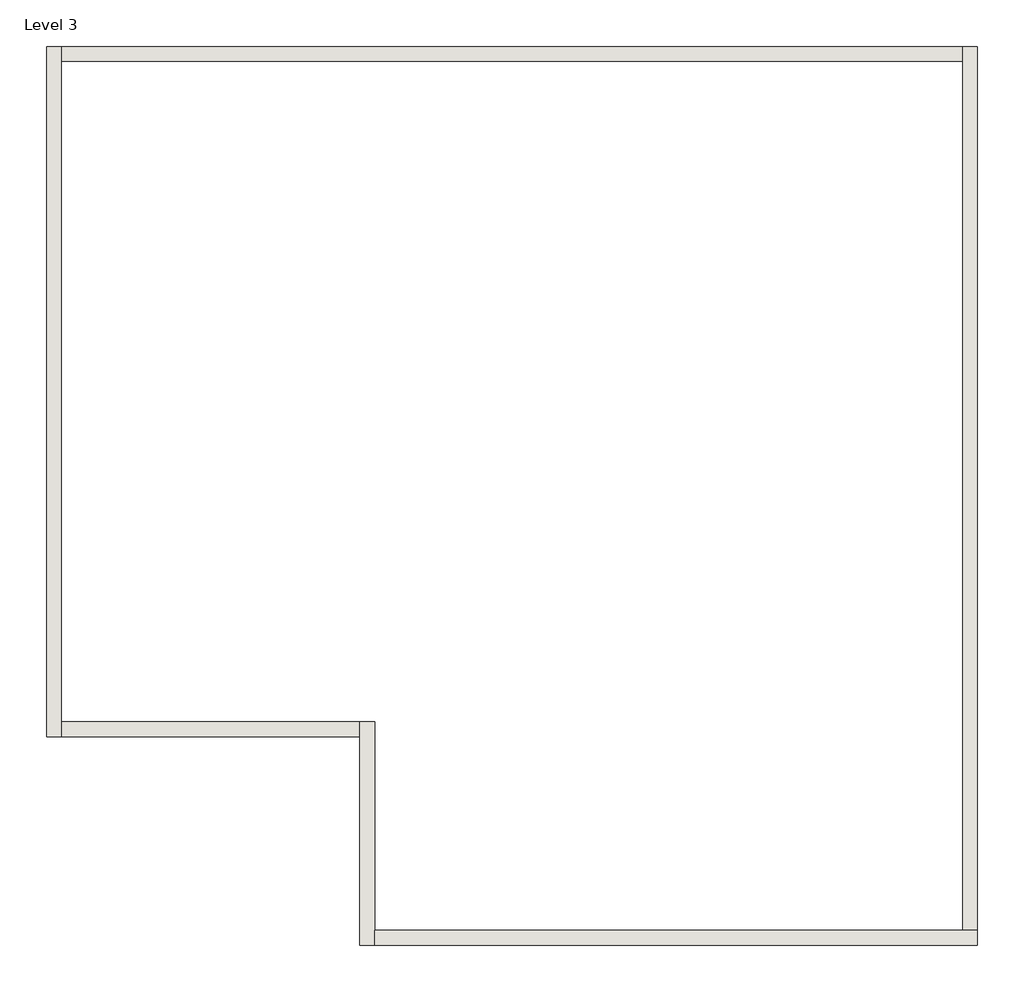
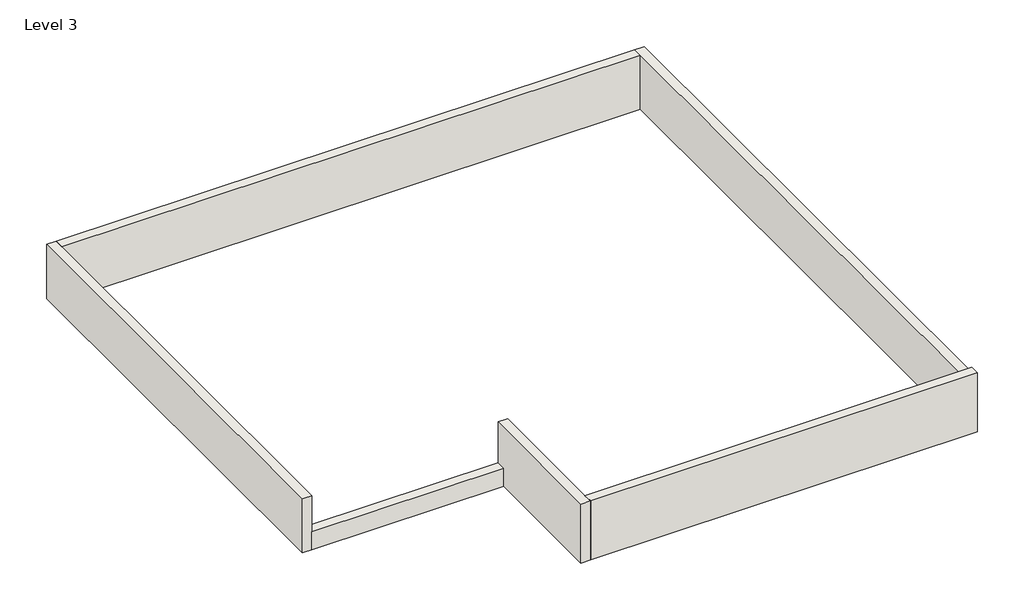
# One storey: 6 walls.
"""IFC4 building model written with IfcOpenShell, lengths in millimetres."""

from ifc_helpers import new_model, si_unit, frame, origin, place, context, project, spatial, polyline, outline, extrude, faceted_brep, element, save

model = new_model("IFC4")

# Units and contexts
model_context = context("Model", 3, world=origin())
ifc_project = project(units=[si_unit("LENGTHUNIT", "METRE", prefix="MILLI")], contexts=[model_context])

# Site, building, storey
site = spatial("IfcSite", under=ifc_project)
building = spatial("IfcBuilding", under=site)
storey = spatial("IfcBuildingStorey", under=building, Name="Level 3", Elevation=3200.4)

# Walls
placement = place(None, origin())
element("IfcWall", 1, ObjectType="6\"", at=placement, inside=storey, context=model_context, shape_type="Brep", body=[
    faceted_brep([(-11281.2102438, 4650.3065419, 3200.4), (-11281.2102438, -2410.8934581, 3200.4), (-11281.2102438, -2410.8934581, 4114.8), (-11281.2102438, 4650.3065419, 4114.8), (-11128.8102438, 4650.3065419, 3200.4), (-11128.8102438, 4650.3065419, 4114.8), (-11128.8102438, 4497.9065419, 4114.8), (-11128.8102438, -2410.8934581, 4114.8), (-11128.8102438, -2410.8934581, 3505.2), (-11128.8102438, -2410.8934581, 3200.4), (-11128.8102438, -2258.4934581, 3200.4), (-11128.8102438, 4497.9065419, 3200.4)], [[[0, 1, 2, 3]], [[4, 5, 6, 7, 8, 9, 10, 11]], [[1, 0, 4, 11, 10, 9]], [[3, 2, 7, 6, 5]], [[2, 1, 9, 8, 7]], [[0, 3, 5, 4]]]),
])
element("IfcWall", 2, ObjectType="6\"", at=placement, inside=storey, context=model_context, shape_type="SweptSolid", body=[
    extrude(outline(polyline([(-8074.4602438, -2410.8934581), (-11128.8102438, -2410.8934581), (-11128.8102438, -2258.4934581), (-8074.4602438, -2258.4934581), (-8074.4602438, -2410.8934581)])), frame((0.0, 0.0, 3200.4), z_axis=(0.0, 0.0, 1.0), x_axis=(1.0, 0.0, 0.0)), (0.0, 0.0, 1.0), 304.8),
])
element("IfcWall", 3, ObjectType="6\"", at=placement, inside=storey, context=model_context, shape_type="Brep", body=[
    faceted_brep([(-8074.4602438, -2258.4934581, 3200.4), (-8074.4602438, -2410.8934581, 3200.4), (-8074.4602438, -4544.4934581, 3200.4), (-8074.4602438, -4544.4934581, 4193.3524321), (-8074.4602438, -2258.4934581, 4193.3524321), (-8074.4602438, -2258.4934581, 3505.2), (-7922.0602438, -2258.4934581, 3200.4), (-7922.0602438, -2258.4934581, 4193.3524321), (-7922.0602438, -4392.0934581, 4193.3524321), (-7922.0602438, -4544.4934581, 4193.3524321), (-7922.0602438, -4544.4934581, 3200.4), (-7922.0602438, -4392.0934581, 3200.4)], [[[0, 1, 2, 3, 4, 5]], [[6, 7, 8, 9, 10, 11]], [[2, 1, 0, 6, 11, 10]], [[4, 3, 9, 8, 7]], [[3, 2, 10, 9]], [[0, 5, 4, 7, 6]]]),
])
element("IfcWall", 4, ObjectType="6\"", at=placement, inside=storey, context=model_context, shape_type="Brep", body=[
    faceted_brep([(-7922.0602438, -4544.4934581, 3200.4), (-1756.2102438, -4544.4934581, 3200.4), (-1756.2102438, -4544.4934581, 4193.3524321), (-7922.0602438, -4544.4934581, 4193.3524321), (-7922.0602438, -4392.0934581, 3200.4), (-7922.0602438, -4392.0934581, 4193.3524321), (-1756.2102438, -4392.0934581, 4193.3524321), (-1756.2102438, -4392.0934581, 4114.8), (-1756.2102438, -4392.0934581, 3200.4), (-1908.6102438, -4392.0934581, 3200.4)], [[[0, 1, 2, 3]], [[4, 5, 6, 7, 8, 9]], [[1, 0, 4, 9, 8]], [[3, 2, 6, 5]], [[2, 1, 8, 7, 6]], [[0, 3, 5, 4]]]),
])
element("IfcWall", 5, ObjectType="6\"", at=placement, inside=storey, context=model_context, shape_type="Brep", body=[
    faceted_brep([(-1756.2102438, -4392.0934581, 3200.4), (-1756.2102438, 4650.3065419, 3200.4), (-1756.2102438, 4650.3065419, 4114.8), (-1756.2102438, -4392.0934581, 4114.8), (-1908.6102438, -4392.0934581, 3200.4), (-1908.6102438, -4392.0934581, 4114.8), (-1908.6102438, 4497.9065419, 4114.8), (-1908.6102438, 4650.3065419, 4114.8), (-1908.6102438, 4650.3065419, 3200.4), (-1908.6102438, 4497.9065419, 3200.4)], [[[0, 1, 2, 3]], [[4, 5, 6, 7, 8, 9]], [[1, 0, 4, 9, 8]], [[3, 2, 7, 6, 5]], [[0, 3, 5, 4]], [[2, 1, 8, 7]]]),
])
element("IfcWall", 6, ObjectType="6\"", at=placement, inside=storey, context=model_context, shape_type="SweptSolid", body=[
    extrude(outline(polyline([(-11128.8102438, 4650.3065419), (-1908.6102438, 4650.3065419), (-1908.6102438, 4497.9065419), (-11128.8102438, 4497.9065419), (-11128.8102438, 4650.3065419)])), frame((0.0, 0.0, 3200.4), z_axis=(0.0, 0.0, 1.0), x_axis=(1.0, 0.0, 0.0)), (0.0, 0.0, 1.0), 914.4),
])

save(model, "model.ifc")

# Revit data of these elements
# Type "6\""
#   Assembly Code = "B2010"
#   Layers, outside or top first: 0' - 6" "Gypsum Wall Board" (function 1)
# Elements 1, 5, 6 (IfcWall, "6\"")
#   Top Offset = 0' - 0"
#   Base Offset = 0' - 0"
#   Unconnected Height = 3' - 0"
#   wall height = 3' - 0"
#   Phase Created = New Construction
#   Base Constraint = Level 3
#   Materials on its faces: "Gypsum Wall Board"
# Element 2 (IfcWall, "6\"")
#   Top Offset = 0' - 0"
#   Base Offset = 0' - 0"
#   Unconnected Height = 1' - 0"
#   wall height = 1' - 0"
#   Phase Created = New Construction
#   Base Constraint = Level 3
#   Materials on its faces: "Gypsum Wall Board"
# Elements 3, 4 (IfcWall, "6\"")
#   Top Offset = 0' - 0"
#   Base Offset = 0' - 0"
#   Unconnected Height = 3' - 3.09262"
#   wall height = 3' - 3.09262"
#   Phase Created = New Construction
#   Base Constraint = Level 3
#   Materials on its faces: "Gypsum Wall Board"
# Materials
#   "Gypsum Wall Board": class "Generic", colour RGB 127 127 127, transparency 0, Description = "Gypsum Wall Board", Cost = 0
